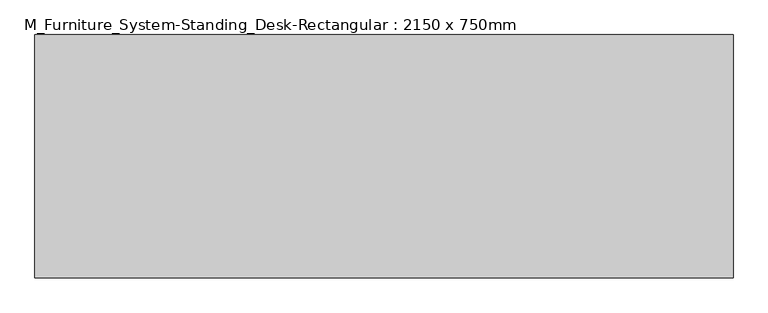
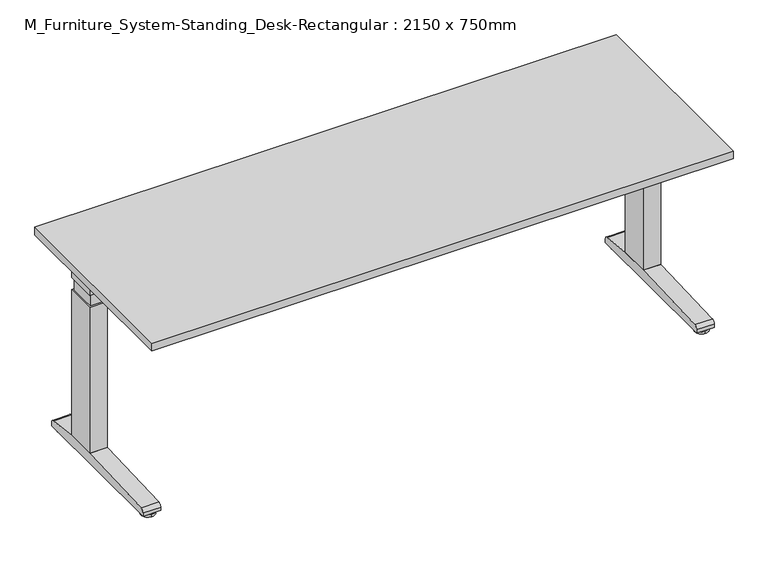
"""IFC4 building model written with IfcOpenShell, lengths in millimetres: furniture geometry, M_Furniture_System-Standing_Desk-Rectangular : 2150 x 750mm."""

from ifc_helpers import new_model, si_unit, point, frame, frame_2d, origin, place, context, project, spatial, polyline, circle_curve, trimmed, segment, composite_curve, outline, extrude, source, transform, mapped, element, save
from ifc_brep_helpers import plane_surface, cylinder_surface, advanced_brep


def m_furniture_system_standing_desk_rectangular_2150_x_750mm_604a6be1(model_context):
    return source(origin(), model_context, "Body", "SolidModel", [
        advanced_brep(
        [(50.8, -610.3, 0.0), (50.8, -661.1, 0.0), (50.8, -635.7, 0.0), (50.8, -610.3, 8.4666667), (50.8, -661.1, 8.4666667), (50.8, -631.4666667, 8.4666667), (50.8, -639.9333333, 8.4666667), (50.8, -631.4666667, 12.7), (50.8, -639.9333333, 12.7), (50.8, -635.7, 12.7)],
        [
            (0, 1, circle_curve(frame((50.8, -635.7, 0.0), z_axis=(0.0, 0.0, -1.0), x_axis=(0.0, -1.0000000000000004, 0.0)), 25.4)),
            (1, 2),
            (2, 0),
            (1, 0, circle_curve(frame((50.8, -635.7, 0.0), z_axis=(0.0, 0.0, -1.0), x_axis=(0.0, -1.0000000000000004, 0.0)), 25.4)),
            (3, 4, circle_curve(frame((50.8, -635.7, 8.4666667), z_axis=(0.0, 0.0, -1.0), x_axis=(0.0, -1.0000000000000004, 0.0)), 25.4)),
            (4, 1),
            (0, 3),
            (4, 3, circle_curve(frame((50.8, -635.7, 8.4666667), z_axis=(0.0, 0.0, -1.0), x_axis=(0.0, -1.0000000000000004, 0.0)), 25.4)),
            (5, 6, circle_curve(frame((50.8, -635.7, 8.4666667), z_axis=(0.0, 0.0, -1.0), x_axis=(0.0, -1.0000000000000004, 0.0)), 4.2333333)),
            (6, 4),
            (3, 5),
            (6, 5, circle_curve(frame((50.8, -635.7, 8.4666667), z_axis=(0.0, 0.0, -1.0), x_axis=(0.0, -1.0000000000000004, 0.0)), 4.2333333)),
            (7, 8, circle_curve(frame((50.8, -635.7, 12.7), z_axis=(0.0, 0.0, -1.0), x_axis=(0.0, -1.0000000000000004, 0.0)), 4.2333333)),
            (8, 6),
            (5, 7),
            (8, 7, circle_curve(frame((50.8, -635.7, 12.7), z_axis=(0.0, 0.0, -1.0), x_axis=(0.0, -1.0000000000000004, 0.0)), 4.2333333)),
            (9, 8),
            (7, 9),
        ],
        [
            plane_surface(frame((50.8, -635.7, 0.0), z_axis=(0.0, 0.0, -1.0), x_axis=(0.0, -1.0, 0.0))),
            cylinder_surface(frame((50.8, -635.7, 69.85), z_axis=(0.0, 0.0, 1.0), x_axis=(0.0, -1.0000000000000004, 0.0)), 25.4),
            plane_surface(frame((50.8, -635.7, 8.4666667), z_axis=(0.0, 0.0, 1.0), x_axis=(0.0, -1.0, 0.0))),
            cylinder_surface(frame((50.8, -635.7, 69.85), z_axis=(0.0, 0.0, 1.0), x_axis=(0.0, -1.0000000000000004, 0.0)), 4.2333333),
            plane_surface(frame((50.8, -635.7, 12.7), z_axis=(0.0, 0.0, 1.0), x_axis=(0.0, -1.0, 0.0))),
        ],
        [
            (0, [[1, 2, 3]]),
            (0, [[4, -3, -2]]),
            (1, [[5, 6, -1, 7]]),
            (1, [[8, -7, -4, -6]]),
            (2, [[9, 10, -5, 11]]),
            (2, [[12, -11, -8, -10]]),
            (3, [[13, 14, -9, 15]]),
            (3, [[16, -15, -12, -14]]),
            (4, [[17, -13, 18]]),
            (4, [[-18, -16, -17]]),
        ],
    ),
        advanced_brep(
        [(50.8, -127.0, 0.0), (50.8, -76.2, 0.0), (50.8, -76.2, 8.4666667), (50.8, -127.0, 8.4666667), (50.8, -97.3666667, 8.4666667), (50.8, -105.8333333, 8.4666667), (50.8, -97.3666667, 12.7), (50.8, -105.8333333, 12.7), (50.8, -101.6, 12.7), (50.8, -101.6, 0.0)],
        [
            (0, 1, circle_curve(frame((50.8, -101.6, 0.0), z_axis=(0.0, 0.0, 1.0), x_axis=(0.0, 1.0000000000000004, 0.0)), 25.4)),
            (1, 2),
            (2, 3, circle_curve(frame((50.8, -101.6, 8.4666667), z_axis=(0.0, 0.0, -1.0), x_axis=(0.0, 1.0000000000000004, 0.0)), 25.4)),
            (3, 0),
            (1, 0, circle_curve(frame((50.8, -101.6, 0.0), z_axis=(0.0, 0.0, 1.0), x_axis=(0.0, 1.0000000000000004, 0.0)), 25.4)),
            (3, 2, circle_curve(frame((50.8, -101.6, 8.4666667), z_axis=(0.0, 0.0, -1.0), x_axis=(0.0, 1.0000000000000004, 0.0)), 25.4)),
            (2, 4),
            (4, 5, circle_curve(frame((50.8, -101.6, 8.4666667), z_axis=(0.0, 0.0, -1.0), x_axis=(0.0, 1.0000000000000004, 0.0)), 4.2333333)),
            (5, 3),
            (5, 4, circle_curve(frame((50.8, -101.6, 8.4666667), z_axis=(0.0, 0.0, -1.0), x_axis=(0.0, 1.0000000000000004, 0.0)), 4.2333333)),
            (4, 6),
            (6, 7, circle_curve(frame((50.8, -101.6, 12.7), z_axis=(0.0, 0.0, -1.0), x_axis=(0.0, 1.0000000000000004, 0.0)), 4.2333333)),
            (7, 5),
            (7, 6, circle_curve(frame((50.8, -101.6, 12.7), z_axis=(0.0, 0.0, -1.0), x_axis=(0.0, 1.0000000000000004, 0.0)), 4.2333333)),
            (6, 8),
            (8, 7),
            (9, 1),
            (0, 9),
        ],
        [
            cylinder_surface(frame((50.8, -101.6, 114.3), z_axis=(0.0, 0.0, -1.0), x_axis=(0.0, 1.0000000000000004, 0.0)), 25.4),
            plane_surface(frame((50.8, -101.6, 8.4666667), z_axis=(0.0, 0.0, 1.0), x_axis=(0.0, 1.0, 0.0))),
            cylinder_surface(frame((50.8, -101.6, 114.3), z_axis=(0.0, 0.0, -1.0), x_axis=(0.0, 1.0000000000000004, 0.0)), 4.2333333),
            plane_surface(frame((50.8, -101.6, 12.7), z_axis=(0.0, 0.0, 1.0), x_axis=(0.0, 1.0, 0.0))),
            plane_surface(frame((50.8, -101.6, 0.0), z_axis=(0.0, 0.0, -1.0), x_axis=(0.0, 1.0, 0.0))),
        ],
        [
            (0, [[1, 2, 3, 4]]),
            (0, [[5, -4, 6, -2]]),
            (1, [[-3, 7, 8, 9]]),
            (1, [[-6, -9, 10, -7]]),
            (2, [[-8, 11, 12, 13]]),
            (2, [[-10, -13, 14, -11]]),
            (3, [[-12, 15, 16]]),
            (3, [[-14, -16, -15]]),
            (4, [[17, -1, 18]]),
            (4, [[-18, -5, -17]]),
        ],
    ),
        extrude(outline(polyline([(83.3, -318.2), (18.3, -318.2), (18.3, -203.2), (83.3, -203.2), (83.3, -318.2)])), frame((0.0, 0.0, 669.2), z_axis=(0.0, 0.0, 1.0), x_axis=(1.0, 0.0, 0.0)), (0.0, 0.0, 1.0), 50.8),
        extrude(outline(polyline([(76.95, -311.85), (24.65, -311.85), (24.65, -209.55), (76.95, -209.55), (76.95, -311.85)])), frame((0.0, 0.0, 622.3), z_axis=(0.0, 0.0, 1.0), x_axis=(1.0, 0.0, 0.0)), (0.0, 0.0, 1.0), 46.9),
        extrude(outline(composite_curve([segment(polyline([(-661.1, 12.7), (-661.1, 25.8616628)]), True, "CONTINUOUS"), segment(trimmed(circle_curve(frame_2d((-648.4, 25.8616628)), 12.7), [point((-661.1, 25.8616628))], [point((-648.8700481, 38.5529612))], False, "CARTESIAN"), True, "CONTINUOUS"), segment(polyline([(-648.8700481, 38.5529612), (-318.2, 50.8), (-203.2, 50.8), (-87.6363028, 39.2436303)]), True, "CONTINUOUS"), segment(trimmed(circle_curve(frame_2d((-88.9, 26.606658)), 12.7), [point((-87.6363028, 39.2436303))], [point((-76.2, 26.606658))], False, "CARTESIAN"), True, "CONTINUOUS"), segment(polyline([(-76.2, 26.606658), (-76.2, 12.7), (-661.1, 12.7)]), True, "CONTINUOUS")], self_intersect=False)), frame((18.3, 0.0, 0.0), z_axis=(1.0, 0.0, 0.0), x_axis=(0.0, 1.0, 0.0)), (0.0, 0.0, 1.0), 65.0),
        extrude(outline(polyline([(83.3, -318.2), (18.3, -318.2), (18.3, -203.2), (83.3, -203.2), (83.3, -318.2)])), frame((0.0, 0.0, 50.8), z_axis=(0.0, 0.0, 1.0), x_axis=(1.0, 0.0, 0.0)), (0.0, 0.0, 1.0), 571.5),
        advanced_brep(
        [(2099.2, -610.3, 0.0), (2099.2, -661.1, 0.0), (2099.2, -635.7, 0.0), (2099.2, -610.3, 8.4666667), (2099.2, -661.1, 8.4666667), (2099.2, -631.4666667, 8.4666667), (2099.2, -639.9333333, 8.4666667), (2099.2, -631.4666667, 12.7), (2099.2, -639.9333333, 12.7), (2099.2, -635.7, 12.7)],
        [
            (0, 1, circle_curve(frame((2099.2, -635.7, 0.0), z_axis=(0.0, 0.0, -1.0), x_axis=(0.0, -1.0, 0.0)), 25.4)),
            (1, 2),
            (2, 0),
            (1, 0, circle_curve(frame((2099.2, -635.7, 0.0), z_axis=(0.0, 0.0, -1.0), x_axis=(0.0, -1.0, 0.0)), 25.4)),
            (3, 4, circle_curve(frame((2099.2, -635.7, 8.4666667), z_axis=(0.0, 0.0, -1.0), x_axis=(0.0, -1.0, 0.0)), 25.4)),
            (4, 1),
            (0, 3),
            (4, 3, circle_curve(frame((2099.2, -635.7, 8.4666667), z_axis=(0.0, 0.0, -1.0), x_axis=(0.0, -1.0, 0.0)), 25.4)),
            (5, 6, circle_curve(frame((2099.2, -635.7, 8.4666667), z_axis=(0.0, 0.0, -1.0), x_axis=(0.0, -1.0, 0.0)), 4.2333333)),
            (6, 4),
            (3, 5),
            (6, 5, circle_curve(frame((2099.2, -635.7, 8.4666667), z_axis=(0.0, 0.0, -1.0), x_axis=(0.0, -1.0, 0.0)), 4.2333333)),
            (7, 8, circle_curve(frame((2099.2, -635.7, 12.7), z_axis=(0.0, 0.0, -1.0), x_axis=(0.0, -1.0, 0.0)), 4.2333333)),
            (8, 6),
            (5, 7),
            (8, 7, circle_curve(frame((2099.2, -635.7, 12.7), z_axis=(0.0, 0.0, -1.0), x_axis=(0.0, -1.0, 0.0)), 4.2333333)),
            (9, 8),
            (7, 9),
        ],
        [
            plane_surface(frame((2099.2, -635.7, 0.0), z_axis=(0.0, 0.0, -1.0), x_axis=(0.0, -1.0, 0.0))),
            cylinder_surface(frame((2099.2, -635.7, 69.85), z_axis=(0.0, 0.0, 1.0), x_axis=(0.0, -1.0, 0.0)), 25.4),
            plane_surface(frame((2099.2, -635.7, 8.4666667), z_axis=(0.0, 0.0, 1.0), x_axis=(0.0, -1.0, 0.0))),
            cylinder_surface(frame((2099.2, -635.7, 69.85), z_axis=(0.0, 0.0, 1.0), x_axis=(0.0, -1.0, 0.0)), 4.2333333),
            plane_surface(frame((2099.2, -635.7, 12.7), z_axis=(0.0, 0.0, 1.0), x_axis=(0.0, -1.0, 0.0))),
        ],
        [
            (0, [[1, 2, 3]]),
            (0, [[4, -3, -2]]),
            (1, [[5, 6, -1, 7]]),
            (1, [[8, -7, -4, -6]]),
            (2, [[9, 10, -5, 11]]),
            (2, [[12, -11, -8, -10]]),
            (3, [[13, 14, -9, 15]]),
            (3, [[16, -15, -12, -14]]),
            (4, [[17, -13, 18]]),
            (4, [[-18, -16, -17]]),
        ],
    ),
        advanced_brep(
        [(2099.2, -127.0, 0.0), (2099.2, -76.2, 0.0), (2099.2, -76.2, 8.4666667), (2099.2, -127.0, 8.4666667), (2099.2, -97.3666667, 8.4666667), (2099.2, -105.8333333, 8.4666667), (2099.2, -97.3666667, 12.7), (2099.2, -105.8333333, 12.7), (2099.2, -101.6, 12.7), (2099.2, -101.6, 0.0)],
        [
            (0, 1, circle_curve(frame((2099.2, -101.6, 0.0), z_axis=(0.0, 0.0, 1.0), x_axis=(0.0, 1.0, 0.0)), 25.4)),
            (1, 2),
            (2, 3, circle_curve(frame((2099.2, -101.6, 8.4666667), z_axis=(0.0, 0.0, -1.0), x_axis=(0.0, 1.0, 0.0)), 25.4)),
            (3, 0),
            (1, 0, circle_curve(frame((2099.2, -101.6, 0.0), z_axis=(0.0, 0.0, 1.0), x_axis=(0.0, 1.0, 0.0)), 25.4)),
            (3, 2, circle_curve(frame((2099.2, -101.6, 8.4666667), z_axis=(0.0, 0.0, -1.0), x_axis=(0.0, 1.0, 0.0)), 25.4)),
            (2, 4),
            (4, 5, circle_curve(frame((2099.2, -101.6, 8.4666667), z_axis=(0.0, 0.0, -1.0), x_axis=(0.0, 1.0, 0.0)), 4.2333333)),
            (5, 3),
            (5, 4, circle_curve(frame((2099.2, -101.6, 8.4666667), z_axis=(0.0, 0.0, -1.0), x_axis=(0.0, 1.0, 0.0)), 4.2333333)),
            (4, 6),
            (6, 7, circle_curve(frame((2099.2, -101.6, 12.7), z_axis=(0.0, 0.0, -1.0), x_axis=(0.0, 1.0, 0.0)), 4.2333333)),
            (7, 5),
            (7, 6, circle_curve(frame((2099.2, -101.6, 12.7), z_axis=(0.0, 0.0, -1.0), x_axis=(0.0, 1.0, 0.0)), 4.2333333)),
            (6, 8),
            (8, 7),
            (9, 1),
            (0, 9),
        ],
        [
            cylinder_surface(frame((2099.2, -101.6, 114.3), z_axis=(0.0, 0.0, -1.0), x_axis=(0.0, 1.0, 0.0)), 25.4),
            plane_surface(frame((2099.2, -101.6, 8.4666667), z_axis=(0.0, 0.0, 1.0), x_axis=(0.0, 1.0, 0.0))),
            cylinder_surface(frame((2099.2, -101.6, 114.3), z_axis=(0.0, 0.0, -1.0), x_axis=(0.0, 1.0, 0.0)), 4.2333333),
            plane_surface(frame((2099.2, -101.6, 12.7), z_axis=(0.0, 0.0, 1.0), x_axis=(0.0, 1.0, 0.0))),
            plane_surface(frame((2099.2, -101.6, 0.0), z_axis=(0.0, 0.0, -1.0), x_axis=(0.0, 1.0, 0.0))),
        ],
        [
            (0, [[1, 2, 3, 4]]),
            (0, [[5, -4, 6, -2]]),
            (1, [[-3, 7, 8, 9]]),
            (1, [[-6, -9, 10, -7]]),
            (2, [[-8, 11, 12, 13]]),
            (2, [[-10, -13, 14, -11]]),
            (3, [[-12, 15, 16]]),
            (3, [[-14, -16, -15]]),
            (4, [[17, -1, 18]]),
            (4, [[-18, -5, -17]]),
        ],
    ),
        extrude(outline(polyline([(2131.7, -318.2), (2066.7, -318.2), (2066.7, -203.2), (2131.7, -203.2), (2131.7, -318.2)])), frame((0.0, 0.0, 669.2), z_axis=(0.0, 0.0, 1.0), x_axis=(1.0, 0.0, 0.0)), (0.0, 0.0, 1.0), 50.8),
        extrude(outline(polyline([(2125.35, -311.85), (2073.05, -311.85), (2073.05, -209.55), (2125.35, -209.55), (2125.35, -311.85)])), frame((0.0, 0.0, 622.3), z_axis=(0.0, 0.0, 1.0), x_axis=(1.0, 0.0, 0.0)), (0.0, 0.0, 1.0), 46.9),
        extrude(outline(composite_curve([segment(polyline([(-661.1, 12.7), (-661.1, 25.8616628)]), True, "CONTINUOUS"), segment(trimmed(circle_curve(frame_2d((-648.4, 25.8616628)), 12.7), [point((-661.1, 25.8616628))], [point((-648.8700481, 38.5529612))], False, "CARTESIAN"), True, "CONTINUOUS"), segment(polyline([(-648.8700481, 38.5529612), (-318.2, 50.8), (-203.2, 50.8), (-87.6363028, 39.2436303)]), True, "CONTINUOUS"), segment(trimmed(circle_curve(frame_2d((-88.9, 26.606658)), 12.7), [point((-87.6363028, 39.2436303))], [point((-76.2, 26.606658))], False, "CARTESIAN"), True, "CONTINUOUS"), segment(polyline([(-76.2, 26.606658), (-76.2, 12.7), (-661.1, 12.7)]), True, "CONTINUOUS")], self_intersect=False)), frame((2066.7, 0.0, 0.0), z_axis=(1.0, 0.0, 0.0), x_axis=(0.0, 1.0, 0.0)), (0.0, 0.0, 1.0), 65.0),
        extrude(outline(polyline([(2131.7, -318.2), (2066.7, -318.2), (2066.7, -203.2), (2131.7, -203.2), (2131.7, -318.2)])), frame((0.0, 0.0, 50.8), z_axis=(0.0, 0.0, 1.0), x_axis=(1.0, 0.0, 0.0)), (0.0, 0.0, 1.0), 571.5),
        extrude(outline(polyline([(2150.0, 0.0), (2150.0, -750.0), (0.0, -750.0), (0.0, 0.0), (2150.0, 0.0)])), frame((0.0, 0.0, 720.0), z_axis=(0.0, 0.0, 1.0), x_axis=(1.0, 0.0, 0.0)), (0.0, 0.0, 1.0), 30.0),
    ])


if __name__ == "__main__":
    model = new_model("IFC4")
    model_context = context("Model", 3, world=origin())
    ifc_project = project(units=[si_unit("LENGTHUNIT", "METRE", prefix="MILLI")], contexts=[model_context])
    site = spatial("IfcSite", under=ifc_project)
    building = spatial("IfcBuilding", under=site)
    placement = place(None, origin())
    m_furniture_system_standing_desk_rectangular_2150_x_750mm_shape = m_furniture_system_standing_desk_rectangular_2150_x_750mm_604a6be1(model_context)
    element("IfcFurniture", 1, ObjectType="M_Furniture_System-Standing_Desk-Rectangular : 2150 x 750mm", at=placement, inside=building, context=model_context, shape_type="MappedRepresentation", body=[
        mapped(m_furniture_system_standing_desk_rectangular_2150_x_750mm_shape, transform((0.0, 0.0, 0.0), x_axis=(1.0, 0.0, 0.0), y_axis=(0.0, 1.0, 0.0), z_axis=(0.0, 0.0, 1.0))),
    ])
    save(model, "model.ifc")

# Revit data of these elements
# Type "M_Furniture_System-Standing_Desk-Rectangular : 2150 x 750mm"
#   Type Comments = "2150 x 750mm Rectangular Standing Desk"
#   Thickness = 30 mm
#   Width = 2150 mm
#   Height [instance default] = 750 mm
#   H [instance default] = 755 mm
#   Foot Height [instance default] = 720 mm
#   Depth = 750 mm
#   Work Surface Material [instance default] = Plastic Laminate - White Oak
#   Foot Material [instance default] = Metal - Paint Linen
#   Edge Material [instance default] = Plastic Laminate - Beige - Light - Smooth
#   Model = ""
#   Manufacturer = ""
#   Description = (empty or 0)
#   Default Elevation = 0
# Element 1 (IfcFurniture, "M_Furniture_System-Standing_Desk-Rectangular : 2150 x 750mm")
#   Materials on its faces: "Metal - Paint Linen", "Plastic Laminate - Beige - Light - Smooth", "Plastic Laminate - White Oak"
# Materials
#   "Plastic Laminate - White Oak": class "Wood", colour RGB 197 170 136, transparency 0
#   "Metal - Paint Linen": class "Metal", colour RGB 244 234 229, transparency 0
#   "Plastic Laminate - Beige - Light - Smooth": class "Plastic", colour RGB 215 199 171, transparency 0
